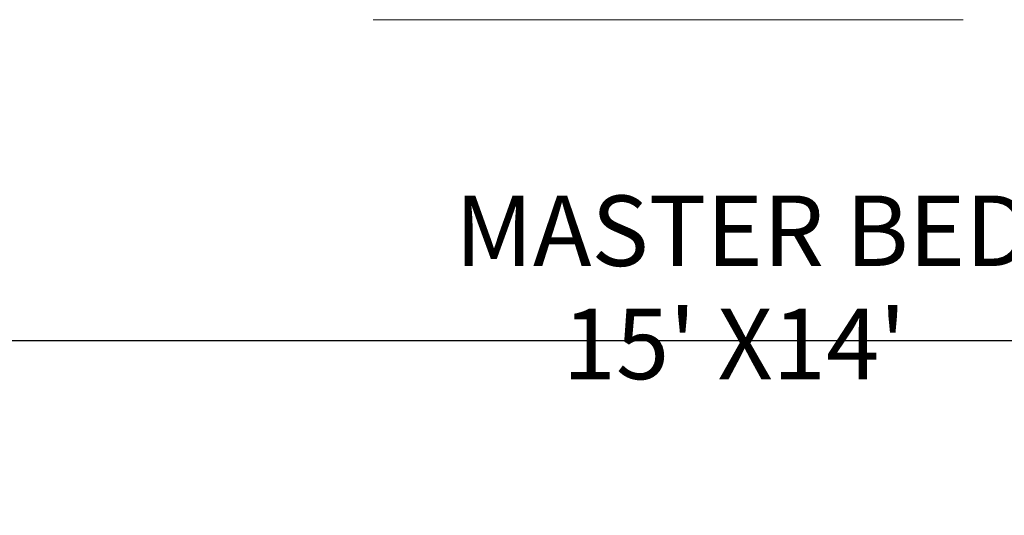
# Model space of a CAD drawing. Units: inches. Extents: x 2025 to 2528, y 1525 to 2336.
# Tile 10 of 18: x 2109 to 2192, y 2167 to 2209. Entities that reach past the tile are written whole.
import ezdxf

# ---------------------------------------------------------------- set-up
doc = ezdxf.new("R2010")
doc.units = ezdxf.units.IN
for name, color, linetype, lineweight in [('A-ANNO-DIMS', 2, 'Continuous', 18), ('A-AREA-IDEN', 7, 'Continuous', 25), ('A-FURN', 8, 'Continuous', 18)]:
    doc.layers.add(name, color=color, linetype=linetype, lineweight=lineweight)
doc.styles.get("Standard").update_dxf_attribs({"font": 'arial.ttf'})
doc.dimstyles.new('Copy of ISO-25', dxfattribs={"dimtxt": 2.5, "dimasz": 2.5, "dimexe": 1.25, "dimexo": 0.625, "dimtad": 1, "dimdec": 1, "dimlunit": 4, "dimtxsty": 'Standard', "dimcen": 2.5, "dimadec": 0, "dimazin": 0, "dimtfac": 1, "dimtdec": 1, "dimtmove": 0, "dimatfit": 3, "dimfxl": 1, "dimarcsym": 0})

# ---------------------------------------------------------------- blocks, each defined once
blk = doc.blocks.new('A$C029D5C69')
blk.add_line((2.0763, 0), (0.5603, 0))
blk = doc.blocks.new('*D77')
at = {"layer": 'A-ANNO-DIMS', "color": 0, "lineweight": -2, "transparency": 16777216}
for p, q in [((2254.388, 2181.412), (2027.213, 2181.412)), ((2028.463, 2153.912), (2028.463, 2178.912)), ((2254.388, 2151.412), (2027.213, 2151.412))]:
    blk.add_line(p, q, dxfattribs=at)
at = {"layer": 'A-ANNO-DIMS', "color": 0, "transparency": 16777216}
for points in [[(2028.046, 2178.912), (2028.88, 2178.912), (2028.463, 2181.412)], [(2028.046, 2153.912), (2028.88, 2153.912), (2028.463, 2151.412)]]:
    blk.add_solid(points, dxfattribs=at)
at = {"layer": 'Defpoints', "color": 0, "transparency": 16777216}
for p in [(2028.463, 2181.412), (2255.013, 2181.412), (2255.013, 2151.412)]:
    blk.add_point(p, dxfattribs=at)
at = {"layer": 'A-ANNO-DIMS', "color": 0, "transparency": 16777216, "insert": (2026.561, 2166.412), "char_height": 2.5, "attachment_point": 5, "rotation": 90}
blk.add_mtext('2\'-6"', dxfattribs=at)
blk = doc.blocks.new('*D80')
at = {"layer": 'A-ANNO-DIMS', "color": 0, "lineweight": -2, "transparency": 16777216}
for p, q in [((2065.388, 2292.412), (2027.213, 2292.412)), ((2028.463, 1566.912), (2028.463, 2289.912)), ((2285.388, 1564.412), (2027.213, 1564.412))]:
    blk.add_line(p, q, dxfattribs=at)
at = {"layer": 'A-ANNO-DIMS', "color": 0, "transparency": 16777216}
for points in [[(2028.046, 2289.912), (2028.88, 2289.912), (2028.463, 2292.412)], [(2028.046, 1566.912), (2028.88, 1566.912), (2028.463, 1564.412)]]:
    blk.add_solid(points, dxfattribs=at)
at = {"layer": 'Defpoints', "color": 0, "transparency": 16777216}
for p in [(2028.463, 2292.412), (2066.013, 2292.412), (2286.013, 1564.412)]:
    blk.add_point(p, dxfattribs=at)
at = {"layer": 'A-ANNO-DIMS', "color": 0, "transparency": 16777216, "insert": (2026.561, 1928.412), "char_height": 2.5, "attachment_point": 5, "rotation": 90}
blk.add_mtext('60\'-8"', dxfattribs=at)

msp = doc.modelspace()

# ---------------------------------------------------------------- block references
at = {"layer": 'A-FURN', "xscale": 33.13032201413296, "yscale": 33.13032201413296, "zscale": 33.13032201413296}
msp.add_blockref('A$C029D5C69', (2120.208, 2208.764), dxfattribs=at)

# ---------------------------------------------------------------- texts
at = {"layer": 'A-AREA-IDEN'}
for s, p in [('MASTER BED ROOM', (2145.715, 2187.791)), ("     15' X14'", (2145.715, 2178.152))]:
    msp.add_text(s, height=6, dxfattribs=at).set_placement(p)

# ---------------------------------------------------------------- dimensions: what is measured, and where the dimension line sits
at = {"layer": 'A-ANNO-DIMS'}
for base, p1, p2, picture, middle in [((2028.463, 2292.412), (2286.013, 1564.412), (2066.013, 2292.412), '*D80', (2026.561, 1928.412)), ((2028.463, 2181.412), (2255.013, 2151.412), (2255.013, 2181.412), '*D77', (2026.561, 2166.412))]:
    dim = msp.add_linear_dim(base=base, p1=p1, p2=p2, angle=90, dimstyle='Copy of ISO-25', override={"dimdec": 1, "dimlfac": 1, "dimrnd": 0, "dimzin": 1, "dimdsep": 46, "dimlunit": 4, "dimfrac": 2}, dxfattribs=at)
    dim.commit()
    dim.dimension.update_dxf_attribs({"geometry": picture, "text_midpoint": middle})

doc.saveas('drawing.dxf')
